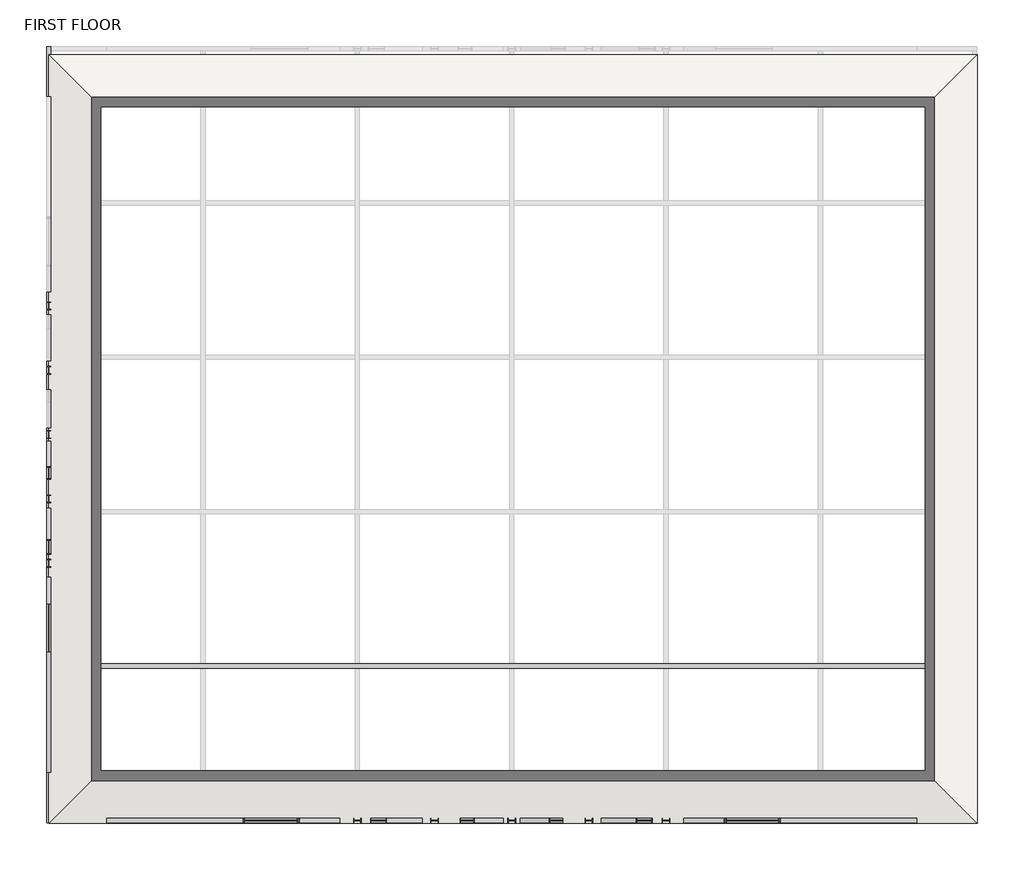
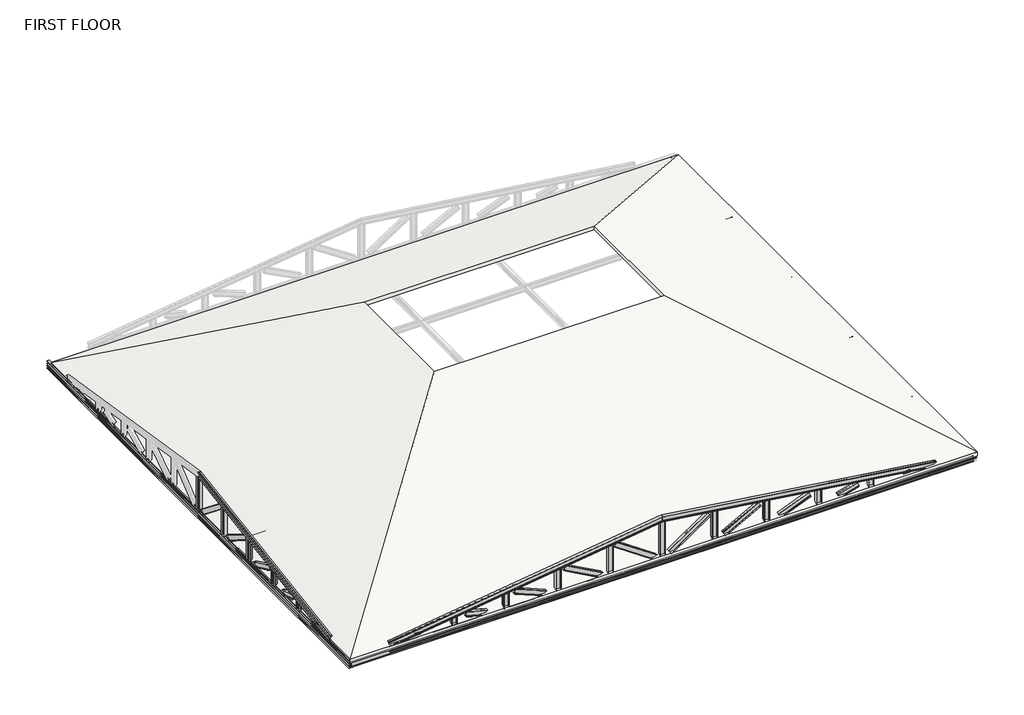
# One storey, part 1 of 2: 40 beams, 1 roof.
"""IFC4 building model written with IfcOpenShell, lengths in millimetres."""

from ifc_helpers import new_model, si_unit, frame, origin, place, context, project, spatial, polyline, circle_curve, ellipse_curve, faceted_brep, transform, mapped, element, save
from ifc_brep_helpers import plane_surface, revolved_surface, advanced_brep
from components import ub_universal_beams_ub305x165x40_0aabe8ba, ub_universal_beams_ub305x165x40_a59d1a35, ub_universal_beams_ub305x165x40_fd314e36, ub_universal_beams_ub305x165x40_8a566974, ub_universal_beams_ub305x165x40_7abb9ae2, ub_universal_beams_ub305x165x40_eb09afc0, ub_universal_beams_ub305x165x40_07ff8ca2, ub_universal_beams_ub305x165x40_bc9e57b7, ub_universal_beams_ub305x165x40_b9dd2748, ub_universal_beams_ub305x165x40_f8f1f307, ub_universal_beams_ub305x165x40_ec3a2bf0, ub_universal_beams_ub305x165x40_23a6c5bf, ub_universal_beams_ub305x165x40_d145b1f7, ub_universal_beams_ub305x165x40_e9518ab5, ub_universal_beams_ub305x165x40_d9098774, ub_universal_beams_ub305x165x40_86e0045c, ub_universal_beams_ub305x165x40_9340f7ff, ub_universal_beams_ub305x165x40_e6c5e72d, ub_universal_beams_ub305x165x40_3f5046e3, ub_universal_beams_ub305x165x40_454c3f6d, ub_universal_beams_ub305x165x40_b4961b4c, ub_universal_beams_ub305x165x40_84569ede, ub_universal_beams_ub305x165x40_9ee690e8, ub_universal_beams_ub305x165x40_49db3f17, ub_universal_beams_ub305x165x40_46279f85, ub_universal_beams_ub305x165x40_94bf3abd, ub_universal_beams_ub305x165x40_babad7d3, ub_universal_beams_ub305x165x40_555319cc, ub_universal_beams_ub305x165x40_491b1046, ub_universal_beams_ub305x165x40_928f9290

model = new_model("IFC4")

# Units and contexts
model_context = context("Model", 3, world=origin())
ifc_project = project(units=[si_unit("LENGTHUNIT", "METRE", prefix="MILLI")], contexts=[model_context])

# Site, building, storey
site = spatial("IfcSite", under=ifc_project)
building = spatial("IfcBuilding", under=site)
storey = spatial("IfcBuildingStorey", under=building, Name="FIRST FLOOR", Elevation=2454.6695361)

# Beams
placement = place(None, origin())
element("IfcBeam", 1, ObjectType="UB-Universal Beams : UB305x165x40", at=placement, inside=storey, context=model_context, shape_type="AdvancedBrep", body=[
    advanced_brep(
    [(15613.2546678, -6274.2308265, 2630.6685888), (15611.8731595, -6274.2308265, 2620.562579), (15611.8731595, -6109.2308265, 2620.562579), (15613.2546678, -6109.2308265, 2630.6685888), (15613.2546678, -6179.8308265, 2630.6685888), (15614.4601016, -6188.7308265, 2639.4865778), (15650.3793185, -6188.7308265, 2902.2428334), (15651.5847522, -6179.8308265, 2911.0608224), (15651.5847522, -6109.2308265, 2911.0608224), (15652.9662606, -6109.2308265, 2921.1668322), (15652.9662606, -6274.2308265, 2921.1668322), (15651.5847522, -6274.2308265, 2911.0608224), (15651.5847522, -6203.6308265, 2911.0608224), (15650.3793185, -6194.7308265, 2902.2428334), (15614.4601016, -6194.7308265, 2639.4865778), (15613.2546678, -6203.6308265, 2630.6685888), (-342.5493858, -6203.6308265, 4811.8535262), (-342.5493858, -6274.2308265, 4811.8535262), (-342.5493858, -6194.7308265, 4820.8363), (-342.5493858, -6194.7308265, 5088.5027722), (-342.5493858, -6203.6308265, 5097.485546), (-342.5493858, -6274.2308265, 5097.485546), (-342.5493858, -6274.2308265, 5107.7804103), (-342.5493858, -6109.2308265, 5107.7804103), (-342.5493858, -6109.2308265, 5097.485546), (-342.5493858, -6179.8308265, 5097.485546), (-342.5493858, -6188.7308265, 5088.5027722), (-342.5493858, -6188.7308265, 4820.8363), (-342.5493858, -6179.8308265, 4811.8535262), (-342.5493858, -6109.2308265, 4811.8535262), (-342.5493858, -6109.2308265, 4801.5586619), (-342.5493858, -6274.2308265, 4801.5586619)],
    [
        (0, 1),
        (1, 2),
        (2, 3),
        (3, 4),
        (4, 5, circle_curve(frame((15614.4601016, -6179.8308265, 2639.4865778), z_axis=(-0.9907852775197102, 0.0, 0.1354419944115965), x_axis=(0.0, 1.0000000000000002, 0.0)), 8.9)),
        (5, 6),
        (6, 7, circle_curve(frame((15650.3793185, -6179.8308265, 2902.2428334), z_axis=(-0.9907852775197102, 0.0, 0.1354419944115965), x_axis=(0.0, 1.0000000000000002, 0.0)), 8.9)),
        (7, 8),
        (8, 9),
        (9, 10),
        (10, 11),
        (11, 12),
        (12, 13, circle_curve(frame((15650.3793185, -6203.6308265, 2902.2428334), z_axis=(-0.9907852775197102, 0.0, 0.1354419944115965), x_axis=(0.0, 1.0000000000000002, 0.0)), 8.9)),
        (13, 14),
        (14, 15, circle_curve(frame((15614.4601016, -6203.6308265, 2639.4865778), z_axis=(-0.9907852775197102, 0.0, 0.1354419944115965), x_axis=(0.0, 1.0000000000000002, 0.0)), 8.9)),
        (15, 0),
        (16, 17),
        (17, 0),
        (15, 16),
        (18, 16, ellipse_curve(frame((-342.5493858, -6203.6308265, 4820.8363), z_axis=(-1.0, 0.0, 0.0), x_axis=(0.0, 0.0, -1.0)), 8.9827738, 8.9)),
        (14, 18),
        (19, 18),
        (13, 19),
        (20, 19, ellipse_curve(frame((-342.5493858, -6203.6308265, 5088.5027722), z_axis=(-1.0, 0.0, 0.0), x_axis=(0.0, 0.0, -1.0)), 8.9827738, 8.9)),
        (12, 20),
        (21, 20),
        (11, 21),
        (22, 21),
        (10, 22),
        (23, 22),
        (9, 23),
        (24, 23),
        (8, 24),
        (25, 24),
        (7, 25),
        (26, 25, ellipse_curve(frame((-342.5493858, -6179.8308265, 5088.5027722), z_axis=(-1.0, 0.0, 0.0), x_axis=(0.0, 0.0, -1.0)), 8.9827738, 8.9)),
        (6, 26),
        (27, 26),
        (5, 27),
        (28, 27, ellipse_curve(frame((-342.5493858, -6179.8308265, 4820.8363), z_axis=(-1.0, 0.0, 0.0), x_axis=(0.0, 0.0, -1.0)), 8.9827738, 8.9)),
        (4, 28),
        (29, 28),
        (3, 29),
        (30, 29),
        (2, 30),
        (31, 30),
        (1, 31),
        (17, 31),
    ],
    [
        plane_surface(frame((15632.41971, -6191.7308265, 2770.8647056), z_axis=(0.9907852775197102, 0.0, -0.1354419944115965), x_axis=(0.1354419944115965, 0.0, 0.9907852775197102))),
        plane_surface(frame((-361.6717543, -6274.2308265, 4814.4675857), z_axis=(0.1354419944115965, 0.0, 0.9907852775197102), x_axis=(0.9907852775197102, 0.0, -0.1354419944115965))),
        revolved_surface(polyline([(15614.460101600422, -6194.7308265, 2639.4865778030694), (-343.75481956224684, -6194.7308265, 4821.001084742412)]), (-360.4663205, -6203.6308265, 4823.2855747), (0.9907852775197102, 0.0, -0.1354419944115965)),
        plane_surface(frame((-360.4663205, -6194.7308265, 4823.2855747), z_axis=(0.0, -1.0000000000000002, 0.0), x_axis=(0.9907852775197102, 0.0, -0.1354419944115965))),
        revolved_surface(polyline([(15650.379318500422, -6194.7308265, 2902.2428334030687), (-343.7548195544014, -6194.7308265, 5088.667556999803)]), (-324.5471036, -6203.6308265, 5086.0418303), (0.9907852775197102, 0.0, -0.1354419944115965)),
        plane_surface(frame((-323.3416699, -6203.6308265, 5094.8598193), z_axis=(-0.1354419944115965, 0.0, -0.9907852775197102), x_axis=(0.9907852775197102, 0.0, -0.1354419944115965))),
        plane_surface(frame((-323.3416699, -6274.2308265, 5094.8598193), z_axis=(0.0, -1.0000000000000002, 0.0), x_axis=(0.9907852775197102, 0.0, -0.1354419944115965))),
        plane_surface(frame((-321.9601615, -6274.2308265, 5104.9658291), z_axis=(0.1354419944115965, 0.0, 0.9907852775197102), x_axis=(0.9907852775197102, 0.0, -0.1354419944115965))),
        plane_surface(frame((-321.9601615, -6109.2308265, 5104.9658291), z_axis=(0.0, 1.0000000000000002, 0.0), x_axis=(0.9907852775197102, 0.0, -0.1354419944115965))),
        plane_surface(frame((-323.3416699, -6109.2308265, 5094.8598193), z_axis=(-0.1354419944115965, 0.0, -0.9907852775197102), x_axis=(0.9907852775197102, 0.0, -0.1354419944115965))),
        revolved_surface(polyline([(15650.379318500422, -6170.9308265, 2902.2428334030687), (-343.7548195544014, -6170.9308265, 5088.667556999803)]), (-324.5471036, -6179.8308265, 5086.0418303), (0.9907852775197102, 0.0, -0.1354419944115965)),
        plane_surface(frame((-324.5471036, -6188.7308265, 5086.0418303), z_axis=(0.0, 1.0000000000000002, 0.0), x_axis=(0.9907852775197102, 0.0, -0.1354419944115965))),
        revolved_surface(polyline([(15614.460101600422, -6170.9308265, 2639.4865778030694), (-343.75481956224684, -6170.9308265, 4821.001084742412)]), (-360.4663205, -6179.8308265, 4823.2855747), (0.9907852775197102, 0.0, -0.1354419944115965)),
        plane_surface(frame((-361.6717543, -6179.8308265, 4814.4675857), z_axis=(0.1354419944115965, 0.0, 0.9907852775197102), x_axis=(0.9907852775197102, 0.0, -0.1354419944115965))),
        plane_surface(frame((-361.6717543, -6109.2308265, 4814.4675857), z_axis=(0.0, 1.0000000000000002, 0.0), x_axis=(0.9907852775197102, 0.0, -0.1354419944115965))),
        plane_surface(frame((-363.0532626, -6109.2308265, 4804.3615759), z_axis=(-0.1354419944115965, 0.0, -0.9907852775197102), x_axis=(0.9907852775197102, 0.0, -0.1354419944115965))),
        plane_surface(frame((-363.0532626, -6274.2308265, 4804.3615759), z_axis=(0.0, -1.0000000000000002, 0.0), x_axis=(0.9907852775197102, 0.0, -0.1354419944115965))),
        plane_surface(frame((-342.5493858, -6191.7308265, 5107.7804103), z_axis=(-1.0, 0.0, 0.0), x_axis=(0.0, 1.0, 0.0))),
    ],
    [
        (0, [[1, 2, 3, 4, 5, 6, 7, 8, 9, 10, 11, 12, 13, 14, 15, 16]]),
        (1, [[17, 18, -16, 19]]),
        (2, [[20, -19, -15, 21]]),
        (3, [[22, -21, -14, 23]]),
        (4, [[24, -23, -13, 25]]),
        (5, [[26, -25, -12, 27]]),
        (6, [[28, -27, -11, 29]]),
        (7, [[30, -29, -10, 31]]),
        (8, [[32, -31, -9, 33]]),
        (9, [[34, -33, -8, 35]]),
        (10, [[36, -35, -7, 37]]),
        (11, [[38, -37, -6, 39]]),
        (12, [[40, -39, -5, 41]]),
        (13, [[42, -41, -4, 43]]),
        (14, [[44, -43, -3, 45]]),
        (15, [[46, -45, -2, 47]]),
        (16, [[48, -47, -1, -18]]),
        (17, [[-17, -20, -22, -24, -26, -28, -30, -32, -34, -36, -38, -40, -42, -44, -46, -48]]),
    ],
),
])
element("IfcBeam", 2, ObjectType="UB-Universal Beams : UB305x165x40", at=placement, inside=storey, context=model_context, shape_type="AdvancedBrep", body=[
    advanced_brep(
    [(-16298.3534395, -6274.2308265, 2630.6685888), (-16298.3534395, -6203.6308265, 2630.6685888), (-16299.5588732, -6194.7308265, 2639.4865778), (-16335.4780901, -6194.7308265, 2902.2428334), (-16336.6835239, -6203.6308265, 2911.0608224), (-16336.6835239, -6274.2308265, 2911.0608224), (-16338.0650322, -6274.2308265, 2921.1668322), (-16338.0650322, -6109.2308265, 2921.1668322), (-16336.6835239, -6109.2308265, 2911.0608224), (-16336.6835239, -6179.8308265, 2911.0608224), (-16335.4780901, -6188.7308265, 2902.2428334), (-16299.5588732, -6188.7308265, 2639.4865778), (-16298.3534395, -6179.8308265, 2630.6685888), (-16298.3534395, -6109.2308265, 2630.6685888), (-16296.9719311, -6109.2308265, 2620.562579), (-16296.9719311, -6274.2308265, 2620.562579), (-342.5493858, -6274.2308265, 4811.8535262), (-342.5493858, -6203.6308265, 4811.8535262), (-342.5493858, -6194.7308265, 4820.8363), (-342.5493858, -6194.7308265, 5088.5027722), (-342.5493858, -6203.6308265, 5097.485546), (-342.5493858, -6274.2308265, 5097.485546), (-342.5493858, -6274.2308265, 5107.7804103), (-342.5493858, -6109.2308265, 5107.7804103), (-342.5493858, -6109.2308265, 5097.485546), (-342.5493858, -6179.8308265, 5097.485546), (-342.5493858, -6188.7308265, 5088.5027722), (-342.5493858, -6188.7308265, 4820.8363), (-342.5493858, -6179.8308265, 4811.8535262), (-342.5493858, -6109.2308265, 4811.8535262), (-342.5493858, -6109.2308265, 4801.5586619), (-342.5493858, -6274.2308265, 4801.5586619)],
    [
        (0, 1),
        (1, 2, circle_curve(frame((-16299.5588732, -6203.6308265, 2639.4865778), z_axis=(0.9907852775197102, 0.0, 0.1354419944115965), x_axis=(0.0, 1.0000000000000002, 0.0)), 8.9)),
        (2, 3),
        (3, 4, circle_curve(frame((-16335.4780901, -6203.6308265, 2902.2428334), z_axis=(0.9907852775197102, 0.0, 0.1354419944115965), x_axis=(0.0, 1.0000000000000002, 0.0)), 8.9)),
        (4, 5),
        (5, 6),
        (6, 7),
        (7, 8),
        (8, 9),
        (9, 10, circle_curve(frame((-16335.4780901, -6179.8308265, 2902.2428334), z_axis=(0.9907852775197102, 0.0, 0.1354419944115965), x_axis=(0.0, 1.0000000000000002, 0.0)), 8.9)),
        (10, 11),
        (11, 12, circle_curve(frame((-16299.5588732, -6179.8308265, 2639.4865778), z_axis=(0.9907852775197102, 0.0, 0.1354419944115965), x_axis=(0.0, 1.0000000000000002, 0.0)), 8.9)),
        (12, 13),
        (13, 14),
        (14, 15),
        (15, 0),
        (0, 16),
        (16, 17),
        (17, 1),
        (17, 18, ellipse_curve(frame((-342.5493858, -6203.6308265, 4820.8363), z_axis=(1.0, 0.0, 0.0), x_axis=(0.0, 0.0, 1.0)), 8.9827738, 8.9)),
        (18, 2),
        (18, 19),
        (19, 3),
        (19, 20, ellipse_curve(frame((-342.5493858, -6203.6308265, 5088.5027722), z_axis=(1.0, 0.0, 0.0), x_axis=(0.0, 0.0, 1.0)), 8.9827738, 8.9)),
        (20, 4),
        (20, 21),
        (21, 5),
        (21, 22),
        (22, 6),
        (22, 23),
        (23, 7),
        (23, 24),
        (24, 8),
        (24, 25),
        (25, 9),
        (25, 26, ellipse_curve(frame((-342.5493858, -6179.8308265, 5088.5027722), z_axis=(1.0, 0.0, 0.0), x_axis=(0.0, 0.0, 1.0)), 8.9827738, 8.9)),
        (26, 10),
        (26, 27),
        (27, 11),
        (27, 28, ellipse_curve(frame((-342.5493858, -6179.8308265, 4820.8363), z_axis=(1.0, 0.0, 0.0), x_axis=(0.0, 0.0, 1.0)), 8.9827738, 8.9)),
        (28, 12),
        (28, 29),
        (29, 13),
        (29, 30),
        (30, 14),
        (30, 31),
        (31, 15),
        (31, 16),
    ],
    [
        plane_surface(frame((-16317.5184817, -6191.7308265, 2770.8647056), z_axis=(-0.9907852775197102, 0.0, -0.1354419944115965), x_axis=(-0.1354419944115965, 0.0, 0.9907852775197102))),
        plane_surface(frame((-16298.3534395, -6274.2308265, 2630.6685888), z_axis=(-0.1354419944115965, 0.0, 0.9907852775197102), x_axis=(0.9907852775197102, 0.0, 0.1354419944115965))),
        revolved_surface(polyline([(-341.3439520373322, -6194.7308265, 4821.001084739342), (-16299.558873253378, -6194.7308265, 2639.486577792703)]), (-16299.5588732, -6203.6308265, 2639.4865778), (0.9907852775197102, 0.0, 0.1354419944115965)),
        plane_surface(frame((-16299.5588732, -6194.7308265, 2639.4865778), z_axis=(0.0, -1.0000000000000002, 0.0), x_axis=(0.9907852775197102, 0.0, 0.1354419944115965))),
        revolved_surface(polyline([(-341.34395204517386, -6194.7308265, 5088.667556996735), (-16335.478090144788, -6194.7308265, 2902.2428333938774)]), (-16335.4780901, -6203.6308265, 2902.2428334), (0.9907852775197102, 0.0, 0.1354419944115965)),
        plane_surface(frame((-16336.6835239, -6203.6308265, 2911.0608224), z_axis=(0.1354419944115965, 0.0, -0.9907852775197102), x_axis=(0.9907852775197102, 0.0, 0.1354419944115965))),
        plane_surface(frame((-16336.6835239, -6274.2308265, 2911.0608224), z_axis=(0.0, -1.0000000000000002, 0.0), x_axis=(0.9907852775197102, 0.0, 0.1354419944115965))),
        plane_surface(frame((-16338.0650322, -6274.2308265, 2921.1668322), z_axis=(-0.1354419944115965, 0.0, 0.9907852775197102), x_axis=(0.9907852775197102, 0.0, 0.1354419944115965))),
        plane_surface(frame((-16338.0650322, -6109.2308265, 2921.1668322), z_axis=(0.0, 1.0000000000000002, 0.0), x_axis=(0.9907852775197102, 0.0, 0.1354419944115965))),
        plane_surface(frame((-16336.6835239, -6109.2308265, 2911.0608224), z_axis=(0.1354419944115965, 0.0, -0.9907852775197102), x_axis=(0.9907852775197102, 0.0, 0.1354419944115965))),
        revolved_surface(polyline([(-341.34395204517386, -6170.9308265, 5088.667556996735), (-16335.478090144788, -6170.9308265, 2902.2428333938774)]), (-16335.4780901, -6179.8308265, 2902.2428334), (0.9907852775197102, 0.0, 0.1354419944115965)),
        plane_surface(frame((-16335.4780901, -6188.7308265, 2902.2428334), z_axis=(0.0, 1.0000000000000002, 0.0), x_axis=(0.9907852775197102, 0.0, 0.1354419944115965))),
        revolved_surface(polyline([(-341.3439520373322, -6170.9308265, 4821.001084739342), (-16299.558873253378, -6170.9308265, 2639.486577792703)]), (-16299.5588732, -6179.8308265, 2639.4865778), (0.9907852775197102, 0.0, 0.1354419944115965)),
        plane_surface(frame((-16298.3534395, -6179.8308265, 2630.6685888), z_axis=(-0.1354419944115965, 0.0, 0.9907852775197102), x_axis=(0.9907852775197102, 0.0, 0.1354419944115965))),
        plane_surface(frame((-16298.3534395, -6109.2308265, 2630.6685888), z_axis=(0.0, 1.0000000000000002, 0.0), x_axis=(0.9907852775197102, 0.0, 0.1354419944115965))),
        plane_surface(frame((-16296.9719311, -6109.2308265, 2620.562579), z_axis=(0.1354419944115965, 0.0, -0.9907852775197102), x_axis=(0.9907852775197102, 0.0, 0.1354419944115965))),
        plane_surface(frame((-16296.9719311, -6274.2308265, 2620.562579), z_axis=(0.0, -1.0000000000000002, 0.0), x_axis=(0.9907852775197102, 0.0, 0.1354419944115965))),
        plane_surface(frame((-342.5493858, -6191.7308265, 5107.7804103), z_axis=(1.0, 0.0, 0.0), x_axis=(0.0, -1.0, 0.0))),
    ],
    [
        (0, [[1, 2, 3, 4, 5, 6, 7, 8, 9, 10, 11, 12, 13, 14, 15, 16]]),
        (1, [[-1, 17, 18, 19]]),
        (2, [[-2, -19, 20, 21]]),
        (3, [[-3, -21, 22, 23]]),
        (4, [[-4, -23, 24, 25]]),
        (5, [[-5, -25, 26, 27]]),
        (6, [[-6, -27, 28, 29]]),
        (7, [[-7, -29, 30, 31]]),
        (8, [[-8, -31, 32, 33]]),
        (9, [[-9, -33, 34, 35]]),
        (10, [[-10, -35, 36, 37]]),
        (11, [[-11, -37, 38, 39]]),
        (12, [[-12, -39, 40, 41]]),
        (13, [[-13, -41, 42, 43]]),
        (14, [[-14, -43, 44, 45]]),
        (15, [[-15, -45, 46, 47]]),
        (16, [[-16, -47, 48, -17]]),
        (17, [[-48, -46, -44, -42, -40, -38, -36, -34, -32, -30, -28, -26, -24, -22, -20, -18]]),
    ],
),
])
element("IfcBeam", 3, ObjectType="UB-Universal Beams : UB305x165x40", at=placement, inside=storey, context=model_context, shape_type="AdvancedBrep", body=[
    advanced_brep(
    [(-18713.0493858, -4242.2632481, 2618.4284465), (-18713.0493858, -4240.676504, 2608.3526219), (-18548.0493858, -4240.676504, 2608.3526219), (-18548.0493858, -4242.2632481, 2618.4284465), (-18618.6493858, -4242.2632481, 2618.4284465), (-18627.5493858, -4243.64776, 2627.2200975), (-18627.5493858, -4284.9031052, 2889.1915396), (-18618.6493858, -4286.2876172, 2897.9831906), (-18548.0493858, -4286.2876172, 2897.9831906), (-18548.0493858, -4287.8743612, 2908.0590153), (-18713.0493858, -4287.8743612, 2908.0590153), (-18713.0493858, -4286.2876172, 2897.9831906), (-18642.4493858, -4286.2876172, 2897.9831906), (-18633.5493858, -4284.9031052, 2889.1915396), (-18633.5493858, -4243.64776, 2627.2200975), (-18642.4493858, -4242.2632481, 2618.4284465), (-18642.4493858, 9048.2691735, 4711.4256783), (-18713.0493858, 9048.2691735, 4711.4256783), (-18633.5493858, 9048.2691735, 4720.4353626), (-18633.5493858, 9048.2691735, 4988.9037095), (-18642.4493858, 9048.2691735, 4997.9133939), (-18713.0493858, 9048.2691735, 4997.9133939), (-18713.0493858, 9048.2691735, 5008.2390995), (-18548.0493858, 9048.2691735, 5008.2390995), (-18548.0493858, 9048.2691735, 4997.9133939), (-18618.6493858, 9048.2691735, 4997.9133939), (-18627.5493858, 9048.2691735, 4988.9037095), (-18627.5493858, 9048.2691735, 4720.4353626), (-18618.6493858, 9048.2691735, 4711.4256783), (-18548.0493858, 9048.2691735, 4711.4256783), (-18548.0493858, 9048.2691735, 4701.0999726), (-18713.0493858, 9048.2691735, 4701.0999726)],
    [
        (0, 1),
        (1, 2),
        (2, 3),
        (3, 4),
        (4, 5, circle_curve(frame((-18618.6493858, -4243.64776, 2627.2200975), z_axis=(0.0, 0.9878259507117182, 0.15556314184436523), x_axis=(1.0, 0.0, 0.0)), 8.9)),
        (5, 6),
        (6, 7, circle_curve(frame((-18618.6493858, -4284.9031052, 2889.1915396), z_axis=(0.0, 0.9878259507117182, 0.15556314184436523), x_axis=(1.0, 0.0, 0.0)), 8.9)),
        (7, 8),
        (8, 9),
        (9, 10),
        (10, 11),
        (11, 12),
        (12, 13, circle_curve(frame((-18642.4493858, -4284.9031052, 2889.1915396), z_axis=(0.0, 0.9878259507117182, 0.15556314184436523), x_axis=(1.0, 0.0, 0.0)), 8.9)),
        (13, 14),
        (14, 15, circle_curve(frame((-18642.4493858, -4243.64776, 2627.2200975), z_axis=(0.0, 0.9878259507117182, 0.15556314184436523), x_axis=(1.0, 0.0, 0.0)), 8.9)),
        (15, 0),
        (16, 17),
        (17, 0),
        (15, 16),
        (18, 16, ellipse_curve(frame((-18642.4493858, 9048.2691735, 4720.4353626), z_axis=(0.0, 1.0, 0.0), x_axis=(0.0, 0.0, -1.0)), 9.0096843, 8.9)),
        (14, 18),
        (19, 18),
        (13, 19),
        (20, 19, ellipse_curve(frame((-18642.4493858, 9048.2691735, 4988.9037095), z_axis=(0.0, 1.0, 0.0), x_axis=(0.0, 0.0, -1.0)), 9.0096843, 8.9)),
        (12, 20),
        (21, 20),
        (11, 21),
        (22, 21),
        (10, 22),
        (23, 22),
        (9, 23),
        (24, 23),
        (8, 24),
        (25, 24),
        (7, 25),
        (26, 25, ellipse_curve(frame((-18618.6493858, 9048.2691735, 4988.9037095), z_axis=(0.0, 1.0, 0.0), x_axis=(0.0, 0.0, -1.0)), 9.0096843, 8.9)),
        (6, 26),
        (27, 26),
        (5, 27),
        (28, 27, ellipse_curve(frame((-18618.6493858, 9048.2691735, 4720.4353626), z_axis=(0.0, 1.0, 0.0), x_axis=(0.0, 0.0, -1.0)), 9.0096843, 8.9)),
        (4, 28),
        (29, 28),
        (3, 29),
        (30, 29),
        (2, 30),
        (31, 30),
        (1, 31),
        (17, 31),
    ],
    [
        plane_surface(frame((-18630.5493858, -4264.2754326, 2758.2058186), z_axis=(0.0, -0.9878259507117182, -0.15556314184436523), x_axis=(0.0, -0.15556314184436523, 0.9878259507117182))),
        plane_surface(frame((-18713.0493858, 9070.2719593, 4714.8906839), z_axis=(0.0, -0.15556314184436523, 0.9878259507117182), x_axis=(0.0, -0.9878259507117182, -0.15556314184436523))),
        revolved_surface(polyline([(-18633.549385799997, -4243.6477600714425, 2627.220097518668), (-18633.549385799997, 9049.653685448697, 4720.653396025778)]), (-18642.4493858, 9068.8874473, 4723.6823349), (0.0, -0.9878259507117182, -0.15556314184436523)),
        plane_surface(frame((-18633.5493858, 9068.8874473, 4723.6823349), z_axis=(-1.0, 0.0, 0.0), x_axis=(0.0, -0.9878259507117182, -0.15556314184436523))),
        revolved_surface(polyline([(-18633.549385799997, -4284.903105235333, 2889.1915396243553), (-18633.549385799997, 9049.65368547084, 4989.121742885172)]), (-18642.4493858, 9027.6321021, 4985.653777), (0.0, -0.9878259507117182, -0.15556314184436523)),
        plane_surface(frame((-18642.4493858, 9026.2475902, 4994.445428), z_axis=(0.0, 0.15556314184436523, -0.9878259507117182), x_axis=(0.0, -0.9878259507117182, -0.15556314184436523))),
        plane_surface(frame((-18713.0493858, 9026.2475902, 4994.445428), z_axis=(-1.0, 0.0, 0.0), x_axis=(0.0, -0.9878259507117182, -0.15556314184436523))),
        plane_surface(frame((-18713.0493858, 9024.6608461, 5004.5212527), z_axis=(0.0, -0.15556314184436523, 0.9878259507117182), x_axis=(0.0, -0.9878259507117182, -0.15556314184436523))),
        plane_surface(frame((-18548.0493858, 9024.6608461, 5004.5212527), z_axis=(1.0, 0.0, 0.0), x_axis=(0.0, -0.9878259507117182, -0.15556314184436523))),
        plane_surface(frame((-18548.0493858, 9026.2475902, 4994.445428), z_axis=(0.0, 0.15556314184436523, -0.9878259507117182), x_axis=(0.0, -0.9878259507117182, -0.15556314184436523))),
        revolved_surface(polyline([(-18609.749385799998, -4284.903105235333, 2889.1915396243553), (-18609.749385799998, 9049.65368547084, 4989.121742885172)]), (-18618.6493858, 9027.6321021, 4985.653777), (0.0, -0.9878259507117182, -0.15556314184436523)),
        plane_surface(frame((-18627.5493858, 9027.6321021, 4985.653777), z_axis=(1.0, 0.0, 0.0), x_axis=(0.0, -0.9878259507117182, -0.15556314184436523))),
        revolved_surface(polyline([(-18609.749385799998, -4243.6477600714425, 2627.220097518668), (-18609.749385799998, 9049.653685448697, 4720.653396025778)]), (-18618.6493858, 9068.8874473, 4723.6823349), (0.0, -0.9878259507117182, -0.15556314184436523)),
        plane_surface(frame((-18618.6493858, 9070.2719593, 4714.8906839), z_axis=(0.0, -0.15556314184436523, 0.9878259507117182), x_axis=(0.0, -0.9878259507117182, -0.15556314184436523))),
        plane_surface(frame((-18548.0493858, 9070.2719593, 4714.8906839), z_axis=(1.0, 0.0, 0.0), x_axis=(0.0, -0.9878259507117182, -0.15556314184436523))),
        plane_surface(frame((-18548.0493858, 9071.8587034, 4704.8148592), z_axis=(0.0, 0.15556314184436523, -0.9878259507117182), x_axis=(0.0, -0.9878259507117182, -0.15556314184436523))),
        plane_surface(frame((-18713.0493858, 9071.8587034, 4704.8148592), z_axis=(-1.0, 0.0, 0.0), x_axis=(0.0, -0.9878259507117182, -0.15556314184436523))),
        plane_surface(frame((-18630.5493858, 9048.2691735, 5008.2390995), z_axis=(0.0, 1.0, 0.0), x_axis=(0.0, 0.0, -1.0))),
    ],
    [
        (0, [[1, 2, 3, 4, 5, 6, 7, 8, 9, 10, 11, 12, 13, 14, 15, 16]]),
        (1, [[17, 18, -16, 19]]),
        (2, [[20, -19, -15, 21]]),
        (3, [[22, -21, -14, 23]]),
        (4, [[24, -23, -13, 25]]),
        (5, [[26, -25, -12, 27]]),
        (6, [[28, -27, -11, 29]]),
        (7, [[30, -29, -10, 31]]),
        (8, [[32, -31, -9, 33]]),
        (9, [[34, -33, -8, 35]]),
        (10, [[36, -35, -7, 37]]),
        (11, [[38, -37, -6, 39]]),
        (12, [[40, -39, -5, 41]]),
        (13, [[42, -41, -4, 43]]),
        (14, [[44, -43, -3, 45]]),
        (15, [[46, -45, -2, 47]]),
        (16, [[48, -47, -1, -18]]),
        (17, [[-17, -20, -22, -24, -26, -28, -30, -32, -34, -36, -38, -40, -42, -44, -46, -48]]),
    ],
),
])
ub_universal_beams_ub305x165x40_shape = ub_universal_beams_ub305x165x40_0aabe8ba(model_context)
element("IfcBeam", 4, ObjectType="UB-Universal Beams : UB305x165x40", at=placement, inside=storey, context=model_context, shape_type="MappedRepresentation", body=[
    mapped(ub_universal_beams_ub305x165x40_shape, transform((-18630.5493858, 9048.2691735, 2302.9695361), x_axis=(0.0, -1.0, 0.0), y_axis=(1.0, 0.0, 0.0), z_axis=(0.0, 0.0, 1.0))),
])
element("IfcBeam", 5, ObjectType="UB-Universal Beams : UB305x165x40", at=placement, inside=storey, context=model_context, shape_type="MappedRepresentation", body=[
    mapped(ub_universal_beams_ub305x165x40_shape, transform((-18630.5493858, 9048.2691735, 2454.6695361), x_axis=(0.0, 1.0, 0.0), y_axis=(-1.0, 0.0, 0.0), z_axis=(0.0, 0.0, 1.0))),
])
ub_universal_beams_ub305x165x40_2_shape = ub_universal_beams_ub305x165x40_a59d1a35(model_context)
element("IfcBeam", 6, ObjectType="UB-Universal Beams : UB305x165x40", at=placement, inside=storey, context=model_context, shape_type="MappedRepresentation", body=[
    mapped(ub_universal_beams_ub305x165x40_2_shape, transform((-342.5493858, -95.7308265, 2302.9695361), x_axis=(1.0, 0.0, 0.0), y_axis=(0.0, 1.0, 0.0), z_axis=(0.0, 0.0, 1.0))),
])
element("IfcBeam", 7, ObjectType="UB-Universal Beams : UB305x165x40", at=placement, inside=storey, context=model_context, shape_type="MappedRepresentation", body=[
    mapped(ub_universal_beams_ub305x165x40_2_shape, transform((-342.5493858, -6191.7308265, 2302.9695361), x_axis=(1.0, 0.0, 0.0), y_axis=(0.0, 1.0, 0.0), z_axis=(0.0, 0.0, 1.0))),
])
ub_universal_beams_ub305x165x40_3_shape = ub_universal_beams_ub305x165x40_fd314e36(model_context)
element("IfcBeam", 8, ObjectType="UB-Universal Beams : UB305x165x40", at=placement, inside=storey, context=model_context, shape_type="MappedRepresentation", body=[
    mapped(ub_universal_beams_ub305x165x40_3_shape, transform((-18630.5493858, 9048.2691735, 3654.6695361), x_axis=(0.0, 0.0, 1.0), y_axis=(1.0, 0.0, 0.0), z_axis=(0.0, 1.0, 0.0))),
])
ub_universal_beams_ub305x165x40_4_shape = ub_universal_beams_ub305x165x40_8a566974(model_context)
element("IfcBeam", 9, ObjectType="UB-Universal Beams : UB305x165x40", at=placement, inside=storey, context=model_context, shape_type="MappedRepresentation", body=[
    mapped(ub_universal_beams_ub305x165x40_4_shape, transform((-18630.5493858, 6508.2691735, 3454.6695361), x_axis=(0.0, 0.0, 1.0), y_axis=(1.0, 0.0, 0.0), z_axis=(0.0, 1.0, 0.0))),
])
ub_universal_beams_ub305x165x40_5_shape = ub_universal_beams_ub305x165x40_7abb9ae2(model_context)
element("IfcBeam", 10, ObjectType="UB-Universal Beams : UB305x165x40", at=placement, inside=storey, context=model_context, shape_type="MappedRepresentation", body=[
    mapped(ub_universal_beams_ub305x165x40_5_shape, transform((-18630.5493858, 3968.2691735, 3254.6695361), x_axis=(0.0, 0.0, 1.0), y_axis=(1.0, 0.0, 0.0), z_axis=(0.0, 1.0, 0.0))),
])
ub_universal_beams_ub305x165x40_6_shape = ub_universal_beams_ub305x165x40_eb09afc0(model_context)
element("IfcBeam", 11, ObjectType="UB-Universal Beams : UB305x165x40", at=placement, inside=storey, context=model_context, shape_type="MappedRepresentation", body=[
    mapped(ub_universal_beams_ub305x165x40_6_shape, transform((-18630.5493858, 1428.2691735, 3054.6695361), x_axis=(0.0, 0.0, 1.0), y_axis=(1.0, 0.0, 0.0), z_axis=(0.0, 1.0, 0.0))),
])
ub_universal_beams_ub305x165x40_7_shape = ub_universal_beams_ub305x165x40_07ff8ca2(model_context)
element("IfcBeam", 12, ObjectType="UB-Universal Beams : UB305x165x40", at=placement, inside=storey, context=model_context, shape_type="MappedRepresentation", body=[
    mapped(ub_universal_beams_ub305x165x40_7_shape, transform((-18630.5493858, -1111.7308265, 2854.6695361), x_axis=(0.0, 0.0, 1.0), y_axis=(1.0, 0.0, 0.0), z_axis=(0.0, 1.0, 0.0))),
])
ub_universal_beams_ub305x165x40_8_shape = ub_universal_beams_ub305x165x40_bc9e57b7(model_context)
element("IfcBeam", 13, ObjectType="UB-Universal Beams : UB305x165x40", at=placement, inside=storey, context=model_context, shape_type="MappedRepresentation", body=[
    mapped(ub_universal_beams_ub305x165x40_8_shape, transform((-18630.5493858, -3651.7308265, 2654.6695361), x_axis=(0.0, 0.0, 1.0), y_axis=(1.0, 0.0, 0.0), z_axis=(0.0, 1.0, 0.0))),
])
ub_universal_beams_ub305x165x40_9_shape = ub_universal_beams_ub305x165x40_b9dd2748(model_context)
element("IfcBeam", 14, ObjectType="UB-Universal Beams : UB305x165x40", at=placement, inside=storey, context=model_context, shape_type="MappedRepresentation", body=[
    mapped(ub_universal_beams_ub305x165x40_9_shape, transform((-18630.5493858, 7778.2691735, 3454.6695361), x_axis=(0.0, 0.7856739006278294, -0.6186408666360893), y_axis=(1.0, 0.0, 0.0), z_axis=(0.0, -0.6186408666360893, -0.7856739006278294))),
])
ub_universal_beams_ub305x165x40_10_shape = ub_universal_beams_ub305x165x40_f8f1f307(model_context)
element("IfcBeam", 15, ObjectType="UB-Universal Beams : UB305x165x40", at=placement, inside=storey, context=model_context, shape_type="MappedRepresentation", body=[
    mapped(ub_universal_beams_ub305x165x40_10_shape, transform((-18630.5493858, 5238.2691735, 3254.6695361), x_axis=(0.0, 0.8461215639131363, -0.5329899615200913), y_axis=(1.0, 0.0, 0.0), z_axis=(0.0, -0.5329899615200913, -0.8461215639131363))),
])
ub_universal_beams_ub305x165x40_11_shape = ub_universal_beams_ub305x165x40_ec3a2bf0(model_context)
element("IfcBeam", 16, ObjectType="UB-Universal Beams : UB305x165x40", at=placement, inside=storey, context=model_context, shape_type="MappedRepresentation", body=[
    mapped(ub_universal_beams_ub305x165x40_11_shape, transform((-18630.5493858, 2698.2691735, 3054.6695361), x_axis=(0.0, 0.9041722720767188, -0.42716800255593146), y_axis=(1.0, 0.0, 0.0), z_axis=(0.0, -0.42716800255593146, -0.9041722720767188))),
])
ub_universal_beams_ub305x165x40_12_shape = ub_universal_beams_ub305x165x40_23a6c5bf(model_context)
element("IfcBeam", 17, ObjectType="UB-Universal Beams : UB305x165x40", at=placement, inside=storey, context=model_context, shape_type="MappedRepresentation", body=[
    mapped(ub_universal_beams_ub305x165x40_12_shape, transform((-18630.5493858, 158.2691735, 2854.6695361), x_axis=(0.0, 0.9538094060666068, -0.3004124113595621), y_axis=(1.0, 0.0, 0.0), z_axis=(0.0, -0.3004124113595621, -0.9538094060666068))),
])
ub_universal_beams_ub305x165x40_13_shape = ub_universal_beams_ub305x165x40_d145b1f7(model_context)
element("IfcBeam", 18, ObjectType="UB-Universal Beams : UB305x165x40", at=placement, inside=storey, context=model_context, shape_type="MappedRepresentation", body=[
    mapped(ub_universal_beams_ub305x165x40_13_shape, transform((-18630.5493858, -2381.7308265, 2654.6695361), x_axis=(0.0, 0.987825950711718, -0.15556314184436557), y_axis=(1.0, 0.0, 0.0), z_axis=(0.0, -0.15556314184436557, -0.987825950711718))),
])
ub_universal_beams_ub305x165x40_14_shape = ub_universal_beams_ub305x165x40_e9518ab5(model_context)
element("IfcBeam", 19, ObjectType="UB-Universal Beams : UB305x165x40", at=placement, inside=storey, context=model_context, shape_type="MappedRepresentation", body=[
    mapped(ub_universal_beams_ub305x165x40_14_shape, transform((-342.5493858, -6191.7308265, 2454.6695361), x_axis=(-1.0, 0.0, 0.0), y_axis=(0.0, -1.0, 0.0), z_axis=(0.0, 0.0, 1.0))),
])
ub_universal_beams_ub305x165x40_15_shape = ub_universal_beams_ub305x165x40_d9098774(model_context)
element("IfcBeam", 20, ObjectType="UB-Universal Beams : UB305x165x40", at=placement, inside=storey, context=model_context, shape_type="MappedRepresentation", body=[
    mapped(ub_universal_beams_ub305x165x40_15_shape, transform((-342.5493858, -6191.7308265, 3704.6695361), x_axis=(0.0, 0.0, 1.0), y_axis=(0.0, 1.0, 0.0), z_axis=(-1.0, 0.0, 0.0))),
])
ub_universal_beams_ub305x165x40_16_shape = ub_universal_beams_ub305x165x40_86e0045c(model_context)
element("IfcBeam", 21, ObjectType="UB-Universal Beams : UB305x165x40", at=placement, inside=storey, context=model_context, shape_type="MappedRepresentation", body=[
    mapped(ub_universal_beams_ub305x165x40_16_shape, transform((2705.4506142, -6191.7308265, 3496.3362027), x_axis=(0.0, 0.0, 1.0), y_axis=(0.0, 1.0, 0.0), z_axis=(-1.0, 0.0, 0.0))),
])
element("IfcBeam", 22, ObjectType="UB-Universal Beams : UB305x165x40", at=placement, inside=storey, context=model_context, shape_type="MappedRepresentation", body=[
    mapped(ub_universal_beams_ub305x165x40_16_shape, transform((-3390.5493858, -6191.7308265, 3496.3362027), x_axis=(0.0, 0.0, 1.0), y_axis=(0.0, 1.0, 0.0), z_axis=(-1.0, 0.0, 0.0))),
])
ub_universal_beams_ub305x165x40_17_shape = ub_universal_beams_ub305x165x40_9340f7ff(model_context)
element("IfcBeam", 23, ObjectType="UB-Universal Beams : UB305x165x40", at=placement, inside=storey, context=model_context, shape_type="MappedRepresentation", body=[
    mapped(ub_universal_beams_ub305x165x40_17_shape, transform((5753.4506142, -6191.7308265, 3288.0028694), x_axis=(0.0, 0.0, 1.0), y_axis=(0.0, 1.0, 0.0), z_axis=(-1.0, 0.0, 0.0))),
])
element("IfcBeam", 24, ObjectType="UB-Universal Beams : UB305x165x40", at=placement, inside=storey, context=model_context, shape_type="MappedRepresentation", body=[
    mapped(ub_universal_beams_ub305x165x40_17_shape, transform((-6438.5493858, -6191.7308265, 3288.0028694), x_axis=(0.0, 0.0, 1.0), y_axis=(0.0, 1.0, 0.0), z_axis=(-1.0, 0.0, 0.0))),
])
ub_universal_beams_ub305x165x40_18_shape = ub_universal_beams_ub305x165x40_e6c5e72d(model_context)
element("IfcBeam", 25, ObjectType="UB-Universal Beams : UB305x165x40", at=placement, inside=storey, context=model_context, shape_type="MappedRepresentation", body=[
    mapped(ub_universal_beams_ub305x165x40_18_shape, transform((8801.4506142, -6191.7308265, 3079.6695361), x_axis=(0.0, 0.0, 1.0), y_axis=(0.0, 1.0, 0.0), z_axis=(-1.0, 0.0, 0.0))),
])
element("IfcBeam", 26, ObjectType="UB-Universal Beams : UB305x165x40", at=placement, inside=storey, context=model_context, shape_type="MappedRepresentation", body=[
    mapped(ub_universal_beams_ub305x165x40_18_shape, transform((-9486.5493858, -6191.7308265, 3079.6695361), x_axis=(0.0, 0.0, 1.0), y_axis=(0.0, 1.0, 0.0), z_axis=(-1.0, 0.0, 0.0))),
])
ub_universal_beams_ub305x165x40_19_shape = ub_universal_beams_ub305x165x40_3f5046e3(model_context)
element("IfcBeam", 27, ObjectType="UB-Universal Beams : UB305x165x40", at=placement, inside=storey, context=model_context, shape_type="MappedRepresentation", body=[
    mapped(ub_universal_beams_ub305x165x40_19_shape, transform((11849.4506142, -6191.7308265, 2871.3362027), x_axis=(0.0, 0.0, 1.0), y_axis=(0.0, 1.0, 0.0), z_axis=(-1.0, 0.0, 0.0))),
])
element("IfcBeam", 28, ObjectType="UB-Universal Beams : UB305x165x40", at=placement, inside=storey, context=model_context, shape_type="MappedRepresentation", body=[
    mapped(ub_universal_beams_ub305x165x40_19_shape, transform((-12534.5493858, -6191.7308265, 2871.3362027), x_axis=(0.0, 0.0, 1.0), y_axis=(0.0, 1.0, 0.0), z_axis=(-1.0, 0.0, 0.0))),
])
ub_universal_beams_ub305x165x40_20_shape = ub_universal_beams_ub305x165x40_454c3f6d(model_context)
element("IfcBeam", 29, ObjectType="UB-Universal Beams : UB305x165x40", at=placement, inside=storey, context=model_context, shape_type="MappedRepresentation", body=[
    mapped(ub_universal_beams_ub305x165x40_20_shape, transform((14897.4506142, -6191.7308265, 2663.0028694), x_axis=(0.0, 0.0, 1.0), y_axis=(0.0, 1.0, 0.0), z_axis=(-1.0, 0.0, 0.0))),
])
element("IfcBeam", 30, ObjectType="UB-Universal Beams : UB305x165x40", at=placement, inside=storey, context=model_context, shape_type="MappedRepresentation", body=[
    mapped(ub_universal_beams_ub305x165x40_20_shape, transform((-15582.5493858, -6191.7308265, 2663.0028694), x_axis=(0.0, 0.0, 1.0), y_axis=(0.0, 1.0, 0.0), z_axis=(-1.0, 0.0, 0.0))),
])
ub_universal_beams_ub305x165x40_21_shape = ub_universal_beams_ub305x165x40_b4961b4c(model_context)
element("IfcBeam", 31, ObjectType="UB-Universal Beams : UB305x165x40", at=placement, inside=storey, context=model_context, shape_type="MappedRepresentation", body=[
    mapped(ub_universal_beams_ub305x165x40_21_shape, transform((1181.4506142, -6191.7308265, 3496.3362027), x_axis=(-0.8255773440876049, 0.0, -0.5642889764378324), y_axis=(0.0, 1.0, 0.0), z_axis=(0.5642889764378324, 0.0, -0.8255773440876049))),
])
ub_universal_beams_ub305x165x40_22_shape = ub_universal_beams_ub305x165x40_84569ede(model_context)
element("IfcBeam", 32, ObjectType="UB-Universal Beams : UB305x165x40", at=placement, inside=storey, context=model_context, shape_type="MappedRepresentation", body=[
    mapped(ub_universal_beams_ub305x165x40_22_shape, transform((4229.4506142, -6191.7308265, 3288.0028694), x_axis=(-0.8773963844437883, 0.0, -0.47976617697058205), y_axis=(0.0, 1.0, 0.0), z_axis=(0.47976617697058205, 0.0, -0.8773963844437883))),
])
ub_universal_beams_ub305x165x40_23_shape = ub_universal_beams_ub305x165x40_9ee690e8(model_context)
element("IfcBeam", 33, ObjectType="UB-Universal Beams : UB305x165x40", at=placement, inside=storey, context=model_context, shape_type="MappedRepresentation", body=[
    mapped(ub_universal_beams_ub305x165x40_23_shape, transform((-1866.5493858, -6191.7308265, 3496.3362027), x_axis=(-0.8255773440876035, 0.0, 0.5642889764378343), y_axis=(0.0, 1.0, 0.0), z_axis=(-0.5642889764378343, 0.0, -0.8255773440876035))),
])
ub_universal_beams_ub305x165x40_24_shape = ub_universal_beams_ub305x165x40_49db3f17(model_context)
element("IfcBeam", 34, ObjectType="UB-Universal Beams : UB305x165x40", at=placement, inside=storey, context=model_context, shape_type="MappedRepresentation", body=[
    mapped(ub_universal_beams_ub305x165x40_24_shape, transform((-4914.5493858, -6191.7308265, 3288.0028694), x_axis=(-0.8773963844437909, 0.0, 0.47976617697057744), y_axis=(0.0, 1.0, 0.0), z_axis=(-0.47976617697057744, 0.0, -0.8773963844437909))),
])
ub_universal_beams_ub305x165x40_25_shape = ub_universal_beams_ub305x165x40_46279f85(model_context)
element("IfcBeam", 35, ObjectType="UB-Universal Beams : UB305x165x40", at=placement, inside=storey, context=model_context, shape_type="MappedRepresentation", body=[
    mapped(ub_universal_beams_ub305x165x40_25_shape, transform((7277.4506142, -6191.7308265, 3079.6695361), x_axis=(-0.9252178070888664, 0.0, -0.3794364366342132), y_axis=(0.0, 1.0, 0.0), z_axis=(0.3794364366342132, 0.0, -0.9252178070888664))),
])
ub_universal_beams_ub305x165x40_26_shape = ub_universal_beams_ub305x165x40_94bf3abd(model_context)
element("IfcBeam", 36, ObjectType="UB-Universal Beams : UB305x165x40", at=placement, inside=storey, context=model_context, shape_type="MappedRepresentation", body=[
    mapped(ub_universal_beams_ub305x165x40_26_shape, transform((-7962.5493858, -6191.7308265, 3079.6695361), x_axis=(-0.9252178070888649, 0.0, 0.3794364366342165), y_axis=(0.0, 1.0, 0.0), z_axis=(-0.3794364366342165, 0.0, -0.9252178070888649))),
])
ub_universal_beams_ub305x165x40_27_shape = ub_universal_beams_ub305x165x40_babad7d3(model_context)
element("IfcBeam", 37, ObjectType="UB-Universal Beams : UB305x165x40", at=placement, inside=storey, context=model_context, shape_type="MappedRepresentation", body=[
    mapped(ub_universal_beams_ub305x165x40_27_shape, transform((10325.4506142, -6191.7308265, 2871.3362027), x_axis=(-0.9645980925721763, 0.0, -0.2637243253970309), y_axis=(0.0, 1.0, 0.0), z_axis=(0.2637243253970309, 0.0, -0.9645980925721763))),
])
ub_universal_beams_ub305x165x40_28_shape = ub_universal_beams_ub305x165x40_555319cc(model_context)
element("IfcBeam", 38, ObjectType="UB-Universal Beams : UB305x165x40", at=placement, inside=storey, context=model_context, shape_type="MappedRepresentation", body=[
    mapped(ub_universal_beams_ub305x165x40_28_shape, transform((-11010.5493858, -6191.7308265, 2871.3362027), x_axis=(-0.9645980925721769, 0.0, 0.26372432539702956), y_axis=(0.0, 1.0, 0.0), z_axis=(-0.26372432539702956, 0.0, -0.9645980925721769))),
])
ub_universal_beams_ub305x165x40_29_shape = ub_universal_beams_ub305x165x40_491b1046(model_context)
element("IfcBeam", 39, ObjectType="UB-Universal Beams : UB305x165x40", at=placement, inside=storey, context=model_context, shape_type="MappedRepresentation", body=[
    mapped(ub_universal_beams_ub305x165x40_29_shape, transform((-14058.5493858, -6191.7308265, 2663.0028694), x_axis=(-0.9907852775197101, 0.0, 0.13544199441159602), y_axis=(0.0, 1.0, 0.0), z_axis=(-0.13544199441159602, 0.0, -0.9907852775197101))),
])
ub_universal_beams_ub305x165x40_30_shape = ub_universal_beams_ub305x165x40_928f9290(model_context)
element("IfcBeam", 40, ObjectType="UB-Universal Beams : UB305x165x40", at=placement, inside=storey, context=model_context, shape_type="MappedRepresentation", body=[
    mapped(ub_universal_beams_ub305x165x40_30_shape, transform((13373.4506142, -6191.7308265, 2663.0028694), x_axis=(-0.9907852775197104, 0.0, -0.13544199441159557), y_axis=(0.0, 1.0, 0.0), z_axis=(0.13544199441159557, 0.0, -0.9907852775197104))),
])

# Roof
element("IfcRoof", 41, ObjectType="Generic - 400mm", at=placement, inside=storey, context=model_context, shape_type="Brep", body=[
    faceted_brep([(-18635.5493858, 24043.2691735, 2454.6695361), (18050.4506142, 24043.2691735, 2454.6695361), (6435.3178986, 12428.136458, 9160.6695361), (-7020.4166703, 12428.136458, 9160.6695361), (-18635.5493858, -6296.7308265, 2454.6695361), (-7020.4166703, 5318.4018891, 9160.6695361), (18050.4506142, -6296.7308265, 2454.6695361), (6435.3178986, 5318.4018891, 9160.6695361), (18050.4506142, 24043.2691735, 2685.6096438), (-18635.5493858, 24043.2691735, 2685.6096438), (-7020.4166703, 12428.136458, 9391.6096438), (6435.3178986, 12428.136458, 9391.6096438), (-18635.5493858, -6296.7308265, 2685.6096438), (-7020.4166703, 5318.4018891, 9391.6096438), (18050.4506142, -6296.7308265, 2685.6096438), (6435.3178986, 5318.4018891, 9391.6096438)], [[[0, 1, 2, 3]], [[4, 0, 3, 5]], [[6, 4, 5, 7]], [[1, 6, 7, 2]], [[8, 9, 10, 11]], [[9, 12, 13, 10]], [[12, 14, 15, 13]], [[14, 8, 11, 15]], [[9, 8, 1, 0]], [[12, 9, 0, 4]], [[14, 12, 4, 6]], [[8, 14, 6, 1]], [[3, 10, 13, 5]], [[5, 13, 15, 7]], [[11, 2, 7, 15]], [[10, 3, 2, 11]]]),
])

save(model, "model.ifc")

# Revit data of these elements
# Type "UB-Universal Beams : UB305x165x40"
#   Section Name Key = "UB305X165X40"
#   Width = 16.5 cm
#   Web Thickness = 0.6 cm
#   Web Fillet = 0.89 cm
#   Warping Constant = 164000.0 cm⁶
#   Torsional Moment of Inertia = 14.70 cm⁴
#   Section Area = 51.3 cm²
#   Plastic Modulus weak axis = 142.0 cm³
#   Plastic Modulus strong axis = 623.0 cm³
#   Nominal Weight = 40.2999 kgf/m
#   Moment of Inertia weak axis = 764.00 cm⁴
#   Moment of Inertia strong axis = 8503.00 cm⁴
#   Height = 30.34 cm
#   Flange Thickness = 1.02 cm
#   Elastic Modulus weak axis = 92.6 cm³
#   Elastic Modulus strong axis = 560.0 cm³
#   Centroid Vertical = 15.17 cm
#   Centroid Horizontal = 8.25 cm
#   Bolt Spacing = 9.0 cm
#   Length [instance default] = 1500 mm
#   Structural Material [instance default] = Metal - Steel 43-275
#   Type Comments = ""
#   Assembly Code = ""
# Type "Generic - 400mm"
#   Layers, outside or top first: 200 mm "Roofing, Tile" (function 1)
# Elements 1, 2, 3, 4, 5, 6, 7, 8, 9, 10, 11, 12, 13, 14, 15, 16, 17, 18, 19, 20, 21, 22, 23, 24, 25, 26, 27, 28, 29, 30, 31, 32, 33, 34, 35, 36, 37, 38, 39, 40 (IfcBeam, "UB-Universal Beams : UB305x165x40")
#   Structural Material = Metal - Steel 43-275
#   Phase Created = New Construction
#   Materials on its faces: "Metal - Steel 43-275"
# Element 41 (IfcRoof, "Generic - 400mm")
#   built-in parameter 1001705 = 30.8124 (stored number, unit not read)
#   built-in parameter 1001710 = 33615
#   Phase Created = New Construction
#   Materials on its faces: "Roofing, Tile"
# Materials
#   "Metal - Steel 43-275": class "Metal", colour RGB 247 247 247, transparency 0, Cost = 0
#   "Roofing, Tile": class "Metal", colour RGB 127 127 127, transparency 0, Description = "Clay roofing tile", Cost = 0
